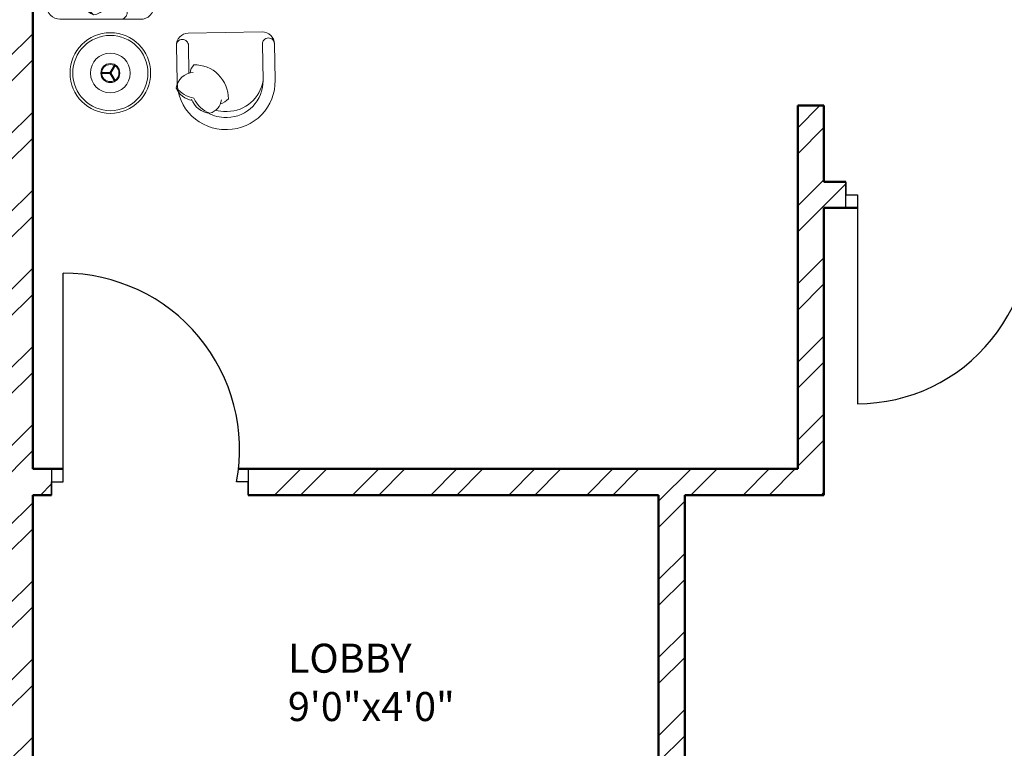
# Model space of a CAD drawing. Units: inches. Extents: x 963 to 2075, y 289 to 2657.
# Tile 82 of 98: x 1511 to 1681, y 2117 to 2243. Entities that reach past the tile are written whole.
import ezdxf

# ---------------------------------------------------------------- set-up
doc = ezdxf.new("R2010")
doc.units = ezdxf.units.IN
for name, color, linetype, lineweight in [('A-AREA-IDEN', 7, 'Continuous', 18), ('A-DOOR', 4, 'Continuous', 25), ('A-FURN', 8, 'Continuous', 18), ('A-WALL', 7, 'Continuous', 50), ('A-WALL-PATT', 8, 'Continuous', 13)]:
    doc.layers.add(name, color=color, linetype=linetype, lineweight=lineweight)
doc.styles.get("Standard").update_dxf_attribs({"font": 'arial.ttf'})

# ---------------------------------------------------------------- blocks, each defined once
blk = doc.blocks.new('ARMCHAIR-A')
at = {"ltscale": 0.03}
blk.add_lwpolyline([(8.89, 17.18), (2.51, 17.18, 0.414214), (0.42, 15.09), (0.42, 8.82, 0.414214), (8.78, 0.46), (8.89, 0.46), (8.99, 0.46, 0.414214), (17.35, 8.82), (17.35, 15.09, 0.414214), (15.26, 17.18), (8.89, 17.18)], format="xyb", dxfattribs=at)
for points in [[(2.51, 8.82), (2.51, 15.09, 0.414214), (1.47, 16.13), (1.47, 16.13, 0.414214), (0.42, 15.09)], [(15.26, 10.28), (15.26, 15.09, -0.414214), (16.31, 16.13), (16.31, 16.13, -0.414214), (17.35, 15.09)], [(15.05, 10.33, 0.165541), (14.41, 11.71, 0.425989), (8.54, 5.73, 0.121523), (9.93, 4.9, -7.115464)], [(14.53, 10.4, -0.356772), (17.52, 7.76, -0.249542), (14.81, 5.59, 9.61688)], [(2.51, 8.82, 0.372719), (8.78, 3.6), (8.89, 3.6)], [(2.51, 8.82, 0.414214), (8.78, 2.55), (8.89, 2.55)], [(17.52, 7.76, -0.14773), (14.47, 5.97, -0.213343), (11.77, 3.34, -0.178662)], [(14.89, 5.83, -0.306663), (11.77, 3.34, -0.30633), (9.74, 5.61, 0.872847)], [(10.77, 3.82, -0.072384), (8.99, 3.6), (8.89, 3.6)], [(12.1, 3.38, -0.130591), (8.99, 2.55), (8.89, 2.55)]]:
    blk.add_lwpolyline(points, format="xyb")
blk = doc.blocks.new('SOFA-3SEAT')
at = {"ltscale": 0.03}
for p, q in [((7.59, 74.33), (6.78, 75.74)), ((7.72, 74.4), (6.9, 75.82)), ((7.59, 74.4), (6.78, 72.99)), ((7.72, 74.33), (6.9, 72.91)), ((7.66, 74.44), (9.29, 74.44)), ((7.66, 74.29), (9.29, 74.29)), ((7.59, 7.12), (6.78, 8.53)), ((7.72, 7.19), (6.9, 8.61)), ((7.59, 7.19), (6.78, 5.78)), ((7.72, 7.12), (6.9, 5.7)), ((7.66, 7.23), (9.29, 7.23)), ((7.66, 7.08), (9.29, 7.08))]:
    blk.add_line(p, q, dxfattribs=at)
blk.add_lwpolyline([(2.44, 16.43, -0.414214), (0.12, 18.74), (0.12, 32.65, -0.414214), (1.28, 33.81, -0.414214), (0.12, 34.97), (0.12, 46.55, -0.414214), (1.28, 47.71, -0.414214), (0.12, 48.87), (0.12, 62.78, -0.414214), (2.44, 65.1), (16.35, 65.1, -0.414214), (18.66, 62.78), (18.66, 18.74, -0.414214), (16.35, 16.43)], format="xyb", close=True, dxfattribs=at)
for points in [[(7.71, 61.62), (5.92, 61.62, -0.414214), (4.76, 62.78), (4.76, 63.94, -0.414214), (5.92, 65.1)], [(7.64, 61.04, -0.356772), (10.56, 64.36, -0.249542), (12.97, 61.35, 9.61688)], [(10.56, 64.36, -0.14773), (12.56, 60.97, -0.213343), (15.48, 57.98, -0.178662)], [(7.71, 61.62, 0.165541), (6.18, 60.9, 0.200231), (8.05, 56.3, 0.121523)], [(12.71, 61.44, -0.306663), (15.48, 57.98, -0.30633), (12.95, 55.72, 0.872847)], [(15.19, 59.18), (15.19, 61.62), (12.91, 61.62, -0.414214)], [(14.03, 60.73), (14.03, 61.16, -0.414214), (14.49, 61.62), (14.72, 61.62, -0.414214), (15.19, 61.16)], [(15.19, 61.16), (15.19, 59.18, -0.414214)], [(7.64, 54.8, -0.356772), (10.56, 58.12, -0.249542), (12.97, 55.11, 9.61688)], [(10.56, 58.12, -0.14773), (12.56, 54.73, -0.213343), (15.48, 51.74, -0.178662)], [(14.03, 54.49), (14.03, 56.09, -0.414214)], [(15.19, 57.25), (15.19, 52.94, -0.414214)], [(7.71, 55.38, 0.165541), (6.18, 54.66, 0.425989), (12.82, 48.15, 0.121523), (13.74, 49.7, -7.115464)], [(12.71, 55.2, -0.306663), (15.48, 51.74, -0.30633), (12.95, 49.48, 0.872847)], [(13.28, 54.97, 0.071865), (13.74, 55.94, -7.115464)], [(15.19, 51.01), (15.19, 48.18, -0.414214), (14.72, 47.71), (14.49, 47.71, -0.414214), (14.03, 48.18), (14.03, 49.84, -0.414214)], [(14.03, 48.87, -0.414214), (12.87, 47.71), (1.28, 47.71, -0.414214)], [(14.03, 46.55, 0.414214), (12.87, 47.71)], [(14.03, 34.97, -0.414214), (12.87, 33.81)], [(14.03, 32.65, 0.414214), (12.87, 33.81), (1.28, 33.81, 0.414214)], [(15.19, 24.27), (15.19, 33.34, 0.414214), (14.72, 33.81), (14.49, 33.81, 0.414214), (14.03, 33.34), (14.03, 25.43, 0.414214)], [(7.71, 19.9, -0.165541), (6.18, 20.62, -0.425989), (12.82, 27.12, -0.121523), (13.74, 25.58, 7.115464)], [(12.71, 20.08, 0.306663), (15.48, 23.54, 0.30633), (12.95, 25.8, -0.872847)], [(10.56, 17.16, 0.14773), (12.56, 20.55, 0.213343), (15.48, 23.54, 0.178662)], [(15.19, 20.37), (15.19, 22.34, 0.414214)], [(7.64, 20.48, 0.356772), (10.56, 17.16, 0.249542), (12.97, 20.17, -9.61688)], [(14.03, 20.79), (14.03, 20.37, 0.414214), (14.49, 19.9), (14.72, 19.9, 0.414214), (15.19, 20.37)], [(5.92, 16.43, -0.414214), (4.76, 17.58), (4.76, 18.74, -0.414214), (5.92, 19.9), (7.71, 19.9)]]:
    blk.add_lwpolyline(points, format="xyb")
for points in [[(15.19, 52.94), (15.19, 57.25)], [(15.19, 24.27), (15.19, 51.01)], [(12.91, 19.9), (15.19, 19.9), (15.19, 22.34)]]:
    blk.add_lwpolyline(points)
blk.add_lwpolyline([(15.19, 47.25), (15.19, 34.27, -0.414214), (14.72, 33.81), (14.49, 33.81, -0.414214), (14.03, 34.27), (14.03, 47.25, -0.414214), (14.49, 47.71), (14.72, 47.71, -0.414214)], format="xyb", close=True)
for centre, radius in [((7.66, 74.37), 6.95), ((7.66, 74.37), 3.42), ((7.66, 74.37), 1.64), ((7.66, 74.37), 1.47), ((7.66, 7.16), 6.95), ((7.66, 7.16), 3.42), ((7.66, 7.16), 1.64), ((7.66, 7.16), 1.47)]:
    blk.add_circle(centre, radius, dxfattribs=at)
for centre in [(7.66, 74.37), (7.66, 7.16)]:
    blk.add_circle(centre, 6.49)

msp = doc.modelspace()

# ---------------------------------------------------------------- hatches: boundary and pattern name
at = {"layer": 'A-WALL-PATT'}
h = msp.add_hatch(dxfattribs=at)
h.set_pattern_fill('ANSI32', color=256)
h.paths.add_polyline_path([(1296.92, 2558.32), (1203.92, 2558.32), (1203.92, 2493.82), (1191.53, 2493.82), (1191.53, 2489.32), (1211.06, 2489.32), (1211.06, 2492.02), (1211.06, 2493.82), (1208.42, 2493.82), (1208.42, 2553.82), (1292.42, 2553.82), (1292.42, 2538.86), (1296.92, 2538.86)])
h.paths.add_polyline_path([(1442.42, 2558.32), (1349.42, 2558.32), (1349.42, 2538.94), (1353.92, 2538.94), (1353.92, 2553.82), (1437.92, 2553.82), (1437.92, 2493.82), (1434.54, 2493.82), (1434.54, 2489.32), (1448.31, 2489.32), (1448.31, 2491.57), (1448.31, 2493.82), (1442.42, 2493.82)])
h.paths.add_polyline_path([(1415.55, 2491.57), (1415.55, 2493.82), (1340.94, 2493.82), (1340.94, 2489.32), (1371.92, 2489.32), (1371.92, 2378.32), (1367.6, 2378.32), (1367.6, 2373.82), (1371.92, 2373.82), (1371.92, 2355.19), (1376.42, 2355.19), (1376.42, 2489.32), (1415.55, 2489.32)])
h.paths.add_polyline_path([(1304.94, 2491.57), (1304.94, 2493.82), (1296.92, 2493.82), (1296.92, 2514.86), (1292.42, 2514.86), (1292.42, 2493.82), (1232.81, 2493.82), (1232.81, 2489.32), (1256.42, 2489.32), (1256.42, 2327.32), (1253.71, 2327.32), (1253.71, 2322.82), (1328.42, 2322.82), (1328.42, 2331.15), (1323.92, 2331.15), (1323.92, 2327.32), (1260.92, 2327.32), (1260.92, 2373.82), (1323.92, 2373.82), (1323.92, 2357.81), (1328.42, 2357.81), (1328.42, 2373.82), (1346.01, 2373.82), (1346.01, 2376.07), (1346.01, 2378.32), (1260.92, 2378.32), (1260.92, 2489.32), (1304.94, 2489.32)])
h.paths.add_polyline_path([(1226.65, 2327.32), (1124.42, 2327.32), (1124.42, 2347.45), (1119.92, 2347.45), (1119.92, 2322.82), (1163.42, 2322.82), (1163.42, 2305.43), (1165.67, 2305.43), (1167.92, 2305.43), (1167.92, 2322.82), (1226.65, 2322.82), (1226.65, 2325.07)])
h.paths.add_polyline_path([(1095.92, 2489.32), (1124.42, 2489.32), (1131.53, 2489.32), (1131.53, 2491.57), (1131.53, 2493.82), (1119.92, 2493.82), (1091.42, 2493.82), (1091.42, 2417.32), (1095.92, 2417.32), (1119.92, 2417.32), (1119.92, 2407.45), (1124.42, 2407.45), (1124.42, 2421.82), (1095.92, 2421.82)])
h.paths.add_polyline_path([(1512.92, 2558.32), (1508.42, 2558.32), (1508.42, 2493.82), (1503.4, 2493.82), (1503.4, 2489.32), (1508.42, 2489.32), (1508.42, 2327.32), (1376.42, 2327.32), (1376.42, 2330.27), (1371.92, 2330.27), (1371.92, 2298.74), (1376.42, 2298.74), (1376.42, 2322.82), (1508.42, 2322.82), (1508.42, 2165.32), (1504.26, 2165.32), (1504.26, 2160.82), (1508.42, 2160.82), (1508.42, 2108.32), (1512.92, 2108.32), (1512.92, 2160.82), (1516.18, 2160.82), (1516.18, 2163.07), (1516.18, 2165.32), (1512.92, 2165.32), (1512.92, 2322.82), (1644.92, 2322.82), (1644.92, 2298.74), (1649.42, 2298.74), (1649.42, 2322.82), (1649.42, 2330.94), (1647.17, 2330.94), (1644.92, 2330.94), (1644.92, 2327.32), (1512.92, 2327.32), (1512.92, 2489.32), (1516.76, 2489.32), (1516.76, 2491.57), (1516.76, 2493.82), (1512.92, 2493.82)])
h.paths.add_polyline_path([(1671.92, 2558.32), (1578.92, 2558.32), (1578.92, 2493.82), (1573.53, 2493.82), (1573.53, 2489.32), (1586.54, 2489.32), (1586.54, 2491.57), (1586.54, 2493.82), (1583.42, 2493.82), (1583.42, 2553.82), (1667.42, 2553.82), (1667.42, 2541.11), (1671.92, 2541.11)])
h.paths.add_polyline_path([(1681.26, 2493.82), (1671.92, 2493.82), (1671.92, 2517.11), (1667.42, 2517.11), (1667.42, 2493.82), (1610.22, 2493.82), (1610.22, 2489.32), (1644.92, 2489.32), (1644.92, 2357.87), (1649.42, 2357.87), (1649.42, 2373.82), (1652.2, 2373.82), (1652.2, 2375.83), (1652.2, 2378.32), (1649.42, 2378.32), (1649.42, 2489.32), (1681.26, 2489.32), (1681.26, 2491.57)])
h.paths.add_polyline_path([(1821.92, 2558.32), (1728.92, 2558.32), (1728.92, 2541), (1733.42, 2541), (1733.42, 2553.82), (1817.42, 2553.82), (1817.42, 2493.82), (1813.51, 2493.82), (1813.51, 2489.32), (1830.08, 2489.32), (1830.08, 2491.57), (1830.08, 2493.82), (1821.92, 2493.82)])
h.paths.add_polyline_path([(1794.24, 2493.82), (1717.26, 2493.82), (1717.26, 2489.32), (1760.42, 2489.32), (1760.42, 2378.32), (1674.4, 2378.32), (1674.4, 2373.82), (1692.92, 2373.82), (1692.92, 2356.95), (1697.42, 2356.95), (1697.42, 2373.82), (1760.42, 2373.82), (1760.42, 2327.32), (1697.42, 2327.32), (1697.42, 2333.34), (1692.92, 2333.34), (1692.92, 2322.82), (1768.04, 2322.82), (1768.04, 2325.07), (1768.04, 2327.32), (1764.92, 2327.32), (1764.92, 2489.32), (1794.24, 2489.32)])
h.paths.add_polyline_path([(1733.42, 2517), (1728.92, 2517), (1728.92, 2493.82), (1733.42, 2493.82)], flags=17)
h.paths.add_polyline_path([(1929.92, 2493.82), (1890.08, 2493.82), (1890.08, 2489.32), (1896.92, 2489.32), (1925.42, 2489.32), (1925.42, 2421.82), (1896.92, 2421.82), (1896.92, 2408.32), (1901.42, 2408.32), (1901.42, 2417.32), (1925.42, 2417.32), (1929.92, 2417.32)])
h.paths.add_polyline_path([(1901.42, 2348.32), (1896.92, 2348.32), (1896.92, 2327.32), (1800.42, 2327.32), (1800.42, 2322.82), (1853.42, 2322.82), (1853.42, 2309.45), (1857.92, 2309.45), (1857.92, 2322.82), (1901.42, 2322.82)])
h.paths.add_polyline_path([(1857.92, 2249.45), (1853.42, 2249.45), (1853.42, 2214.82), (1686.31, 2214.82), (1686.31, 2210.32), (1853.42, 2210.32), (1853.42, 2202.13), (1857.92, 2202.13), (1857.92, 2210.32)])
h.paths.add_polyline_path([(1857.92, 2142.13), (1853.42, 2142.13), (1853.42, 2115.42), (1841.42, 2115.42), (1841.42, 2088.53), (1841.42, 2046.95), (1845.92, 2046.95), (1845.92, 2110.92), (1905.92, 2110.92), (1905.92, 2092.52), (1910.42, 2092.52), (1910.42, 2115.42), (1857.92, 2115.42)])
h.paths.add_polyline_path([(1532.44, 1482.34), (1573.46, 1482.34), (1573.46, 1501), (1532.44, 1501)], flags=9)
h.paths.add_polyline_path([(1438.66, 1486.3), (1479.68, 1486.3), (1479.68, 1504.96), (1438.66, 1504.96)], flags=9)
h.paths.add_polyline_path([(1411.22, 1365.31), (1659.14, 1365.31), (1659.14, 1402.4), (1411.22, 1402.4)], flags=9)
h.paths.add_polyline_path([(1185.67, 2296.3), (1248.16, 2296.3), (1248.16, 2314.95), (1185.67, 2314.95)], flags=9)
h.paths.add_polyline_path([(1177.31, 2187.35), (1216.15, 2187.35), (1216.15, 2206.01), (1177.31, 2206.01)], flags=9)
h.paths.add_polyline_path([(1295.1, 1602.08), (1328.26, 1602.08), (1328.26, 1620.74), (1295.1, 1620.74)], flags=9)
h.paths.add_polyline_path([(1525.13, 2005.99), (1558.39, 2005.99), (1558.39, 2024.65), (1525.13, 2024.65)], flags=9)
h.paths.add_polyline_path([(1459.61, 1977.13), (1472.19, 1977.13), (1472.19, 1987.43), (1459.61, 1987.43)], flags=9)
h.paths.add_polyline_path([(1467.81, 2053.68), (1480.02, 2053.68), (1480.02, 2063.98), (1467.81, 2063.98)], flags=9)
h.paths.add_polyline_path([(1555.18, 2119.02), (1584.56, 2119.02), (1584.56, 2137.68), (1555.18, 2137.68)], flags=25)
h.paths.add_polyline_path([(1405.39, 2115.29), (1444.48, 2115.29), (1444.48, 2133.95), (1405.39, 2133.95)], flags=25)
h.paths.add_polyline_path([(1698.48, 2004.26), (1727.69, 2004.26), (1727.69, 2022.92), (1698.48, 2022.92)], flags=9)
h.paths.add_polyline_path([(1612.16, 1972.86), (1629.02, 1972.86), (1629.02, 1983.16), (1612.16, 1983.16)], flags=9)
h.paths.add_polyline_path([(1608.29, 2060.04), (1625.15, 2060.04), (1625.15, 2070.34), (1608.29, 2070.34)], flags=9)
h.paths.add_polyline_path([(1527.95, 1684.4), (1566.79, 1684.4), (1566.79, 1703.06), (1527.95, 1703.06)], flags=9)
h.paths.add_polyline_path([(1422.79, 1683.59), (1461.63, 1683.59), (1461.63, 1702.25), (1422.79, 1702.25)], flags=9)
h.paths.add_polyline_path([(1531.26, 1732.46), (1574.01, 1732.46), (1574.01, 1751.12), (1531.26, 1751.12)], flags=9)
h.paths.add_polyline_path([(1402.87, 1732.85), (1439.8, 1732.85), (1439.8, 1751.5), (1402.87, 1751.5)], flags=9)
h.paths.add_polyline_path([(1243.12, 1923.13), (1281.96, 1923.13), (1281.96, 1941.79), (1243.12, 1941.79)], flags=9)
h.paths.add_polyline_path([(1181.75, 1792.27), (1244.24, 1792.27), (1244.24, 1810.93), (1181.75, 1810.93)], flags=9)
h.paths.add_polyline_path([(1265.82, 1670.3), (1316.07, 1670.3), (1316.07, 1688.96), (1265.82, 1688.96)], flags=9)
h.paths.add_polyline_path([(1140.26, 1676.05), (1179.1, 1676.05), (1179.1, 1694.71), (1140.26, 1694.71)], flags=9)
h.paths.add_polyline_path([(1107.49, 1490.89), (1143.37, 1490.89), (1143.37, 1509.55), (1107.49, 1509.55)], flags=9)
h.paths.add_polyline_path([(1217.58, 1483.9), (1246.74, 1483.9), (1246.74, 1502.56), (1217.58, 1502.56)], flags=9)
h.paths.add_polyline_path([(1389.21, 1486.92), (1418.37, 1486.92), (1418.37, 1505.58), (1389.21, 1505.58)], flags=9)
h.paths.add_polyline_path([(1672.21, 1602.08), (1705.37, 1602.08), (1705.37, 1620.74), (1672.21, 1620.74)], flags=9)
h.paths.add_polyline_path([(1752.08, 1522.64), (1781.24, 1522.64), (1781.24, 1541.3), (1752.08, 1541.3)], flags=9)
h.paths.add_polyline_path([(1848.27, 1491.26), (1884.16, 1491.26), (1884.16, 1509.92), (1848.27, 1509.92)], flags=9)
h.paths.add_polyline_path([(1822.47, 1685.62), (1861.31, 1685.62), (1861.31, 1704.28), (1822.47, 1704.28)], flags=9)
h.paths.add_polyline_path([(1713.19, 1672.23), (1763.44, 1672.23), (1763.44, 1690.89), (1713.19, 1690.89)], flags=9)
h.paths.add_polyline_path([(1736.62, 1790.58), (1799.11, 1790.58), (1799.11, 1809.24), (1736.62, 1809.24)], flags=9)
h.paths.add_polyline_path([(1691.49, 1916.36), (1730.33, 1916.36), (1730.33, 1935.01), (1691.49, 1935.01)], flags=9)
h.paths.add_polyline_path([(1764.87, 1973.92), (1794.31, 1973.92), (1794.31, 1992.58), (1764.87, 1992.58)], flags=9)
h.paths.add_polyline_path([(1767.85, 2034.02), (1797.29, 2034.02), (1797.29, 2052.67), (1767.85, 2052.67)], flags=9)
h.paths.add_polyline_path([(1851.59, 2060.33), (1880.75, 2060.33), (1880.75, 2078.99), (1851.59, 2078.99)], flags=25)
h.paths.add_polyline_path([(1688.49, 2086.87), (1727.33, 2086.87), (1727.33, 2105.53), (1688.49, 2105.53)], flags=9)
h.paths.add_polyline_path([(1537.74, 2293.58), (1580.49, 2293.58), (1580.49, 2312.24), (1537.74, 2312.24)], flags=25)
h.paths.add_polyline_path([(1425.59, 2296.11), (1468.34, 2296.11), (1468.34, 2314.77), (1425.59, 2314.77)], flags=25)
h.paths.add_polyline_path([(1278.52, 2004.18), (1307.72, 2004.18), (1307.72, 2022.84), (1278.52, 2022.84)], flags=9)
h.paths.add_polyline_path([(1193.28, 1973.63), (1222.72, 1973.63), (1222.72, 1992.29), (1193.28, 1992.29)], flags=9)
h.paths.add_polyline_path([(1192.41, 2040.58), (1221.84, 2040.58), (1221.84, 2059.23), (1192.41, 2059.23)], flags=9)
h.paths.add_polyline_path([(1130.6, 1951.39), (1159.76, 1951.39), (1159.76, 1970.05), (1130.6, 1970.05)], flags=9)
h.paths.add_polyline_path([(1132.83, 2052.49), (1161.98, 2052.49), (1161.98, 2071.15), (1132.83, 2071.15)], flags=9)
h.paths.add_polyline_path([(1265.13, 2334.62), (1315.38, 2334.62), (1315.38, 2353.28), (1265.13, 2353.28)], flags=25)
h.paths.add_polyline_path([(1136.74, 2330.79), (1175.58, 2330.79), (1175.58, 2349.44), (1136.74, 2349.44)], flags=9)
h.paths.add_polyline_path([(1287.42, 2417.2), (1320.58, 2417.2), (1320.58, 2435.86), (1287.42, 2435.86)], flags=25)
h.paths.add_polyline_path([(1430.99, 2329.16), (1469.83, 2329.16), (1469.83, 2347.82), (1430.99, 2347.82)], flags=25)
h.paths.add_polyline_path([(1525.42, 2329.21), (1564.26, 2329.21), (1564.26, 2347.87), (1525.42, 2347.87)], flags=25)
h.paths.add_polyline_path([(1684.52, 2382.8), (1717.68, 2382.8), (1717.68, 2401.46), (1684.52, 2401.46)], flags=25)
h.paths.add_polyline_path([(1704.81, 2340.29), (1755.05, 2340.29), (1755.05, 2358.95), (1704.81, 2358.95)], flags=25)
h.paths.add_polyline_path([(1694.11, 2287.76), (1756.6, 2287.76), (1756.6, 2306.41), (1694.11, 2306.41)], flags=9)
h.paths.add_polyline_path([(1815.78, 2329.86), (1854.62, 2329.86), (1854.62, 2348.52), (1815.78, 2348.52)], flags=9)
h.paths.add_polyline_path([(1842.87, 2514.26), (1878.76, 2514.26), (1878.76, 2532.91), (1842.87, 2532.91)], flags=9)
h.paths.add_polyline_path([(1769.51, 2531.45), (1798.67, 2531.45), (1798.67, 2550.1), (1769.51, 2550.1)], flags=25)
h.paths.add_polyline_path([(1594.77, 2518.47), (1623.93, 2518.47), (1623.93, 2537.13), (1594.77, 2537.13)], flags=25)
h.paths.add_polyline_path([(1520.72, 2516.18), (1556.61, 2516.18), (1556.61, 2534.84), (1520.72, 2534.84)], flags=25)
h.paths.add_polyline_path([(1464.46, 2516.69), (1500.34, 2516.69), (1500.34, 2535.35), (1464.46, 2535.35)], flags=25)
h.paths.add_polyline_path([(1365.7, 2528.97), (1394.85, 2528.97), (1394.85, 2547.63), (1365.7, 2547.63)], flags=25)
h.paths.add_polyline_path([(1222.84, 2516.23), (1252, 2516.23), (1252, 2534.89), (1222.84, 2534.89)], flags=25)
h.paths.add_polyline_path([(1104.55, 2509.6), (1140.43, 2509.6), (1140.43, 2528.26), (1104.55, 2528.26)], flags=9)
h = msp.add_hatch(dxfattribs=at)
h.set_pattern_fill('ANSI32', color=256)
h.paths.add_polyline_path([(1335.97, 2212.57), (1335.97, 2214.82), (1167.92, 2214.82), (1167.92, 2245.43), (1163.42, 2245.43), (1163.42, 2210.32), (1163.42, 2194.81), (1167.92, 2194.81), (1167.92, 2210.32), (1335.97, 2210.32)])
h.paths.add_polyline_path([(1532.44, 1482.34), (1573.46, 1482.34), (1573.46, 1501), (1532.44, 1501)], flags=9)
h.paths.add_polyline_path([(1438.66, 1486.3), (1479.68, 1486.3), (1479.68, 1504.96), (1438.66, 1504.96)], flags=9)
h.paths.add_polyline_path([(1411.22, 1365.31), (1659.14, 1365.31), (1659.14, 1402.4), (1411.22, 1402.4)], flags=9)
h.paths.add_polyline_path([(1185.67, 2296.3), (1248.16, 2296.3), (1248.16, 2314.95), (1185.67, 2314.95)], flags=9)
h.paths.add_polyline_path([(1177.31, 2187.35), (1216.15, 2187.35), (1216.15, 2206.01), (1177.31, 2206.01)], flags=9)
h.paths.add_polyline_path([(1295.1, 1602.08), (1328.26, 1602.08), (1328.26, 1620.74), (1295.1, 1620.74)], flags=9)
h.paths.add_polyline_path([(1525.13, 2005.99), (1558.39, 2005.99), (1558.39, 2024.65), (1525.13, 2024.65)], flags=9)
h.paths.add_polyline_path([(1459.61, 1977.13), (1472.19, 1977.13), (1472.19, 1987.43), (1459.61, 1987.43)], flags=9)
h.paths.add_polyline_path([(1467.81, 2053.68), (1480.02, 2053.68), (1480.02, 2063.98), (1467.81, 2063.98)], flags=9)
h.paths.add_polyline_path([(1555.18, 2119.02), (1584.56, 2119.02), (1584.56, 2137.68), (1555.18, 2137.68)], flags=9)
h.paths.add_polyline_path([(1405.39, 2115.29), (1444.48, 2115.29), (1444.48, 2133.95), (1405.39, 2133.95)], flags=9)
h.paths.add_polyline_path([(1698.48, 2004.26), (1727.69, 2004.26), (1727.69, 2022.92), (1698.48, 2022.92)], flags=9)
h.paths.add_polyline_path([(1612.16, 1972.86), (1629.02, 1972.86), (1629.02, 1983.16), (1612.16, 1983.16)], flags=9)
h.paths.add_polyline_path([(1608.29, 2060.04), (1625.15, 2060.04), (1625.15, 2070.34), (1608.29, 2070.34)], flags=9)
h.paths.add_polyline_path([(1527.95, 1684.4), (1566.79, 1684.4), (1566.79, 1703.06), (1527.95, 1703.06)], flags=9)
h.paths.add_polyline_path([(1422.79, 1683.59), (1461.63, 1683.59), (1461.63, 1702.25), (1422.79, 1702.25)], flags=9)
h.paths.add_polyline_path([(1531.26, 1732.46), (1574.01, 1732.46), (1574.01, 1751.12), (1531.26, 1751.12)], flags=9)
h.paths.add_polyline_path([(1402.87, 1732.85), (1439.8, 1732.85), (1439.8, 1751.5), (1402.87, 1751.5)], flags=9)
h.paths.add_polyline_path([(1243.12, 1923.13), (1281.96, 1923.13), (1281.96, 1941.79), (1243.12, 1941.79)], flags=9)
h.paths.add_polyline_path([(1181.75, 1792.27), (1244.24, 1792.27), (1244.24, 1810.93), (1181.75, 1810.93)], flags=9)
h.paths.add_polyline_path([(1265.82, 1670.3), (1316.07, 1670.3), (1316.07, 1688.96), (1265.82, 1688.96)], flags=9)
h.paths.add_polyline_path([(1140.26, 1676.05), (1179.1, 1676.05), (1179.1, 1694.71), (1140.26, 1694.71)], flags=9)
h.paths.add_polyline_path([(1107.49, 1490.89), (1143.37, 1490.89), (1143.37, 1509.55), (1107.49, 1509.55)], flags=9)
h.paths.add_polyline_path([(1217.58, 1483.9), (1246.74, 1483.9), (1246.74, 1502.56), (1217.58, 1502.56)], flags=9)
h.paths.add_polyline_path([(1389.21, 1486.92), (1418.37, 1486.92), (1418.37, 1505.58), (1389.21, 1505.58)], flags=9)
h.paths.add_polyline_path([(1672.21, 1602.08), (1705.37, 1602.08), (1705.37, 1620.74), (1672.21, 1620.74)], flags=9)
h.paths.add_polyline_path([(1752.08, 1522.64), (1781.24, 1522.64), (1781.24, 1541.3), (1752.08, 1541.3)], flags=9)
h.paths.add_polyline_path([(1848.27, 1491.26), (1884.16, 1491.26), (1884.16, 1509.92), (1848.27, 1509.92)], flags=9)
h.paths.add_polyline_path([(1822.47, 1685.62), (1861.31, 1685.62), (1861.31, 1704.28), (1822.47, 1704.28)], flags=9)
h.paths.add_polyline_path([(1713.19, 1672.23), (1763.44, 1672.23), (1763.44, 1690.89), (1713.19, 1690.89)], flags=9)
h.paths.add_polyline_path([(1736.62, 1790.58), (1799.11, 1790.58), (1799.11, 1809.24), (1736.62, 1809.24)], flags=9)
h.paths.add_polyline_path([(1691.49, 1916.36), (1730.33, 1916.36), (1730.33, 1935.01), (1691.49, 1935.01)], flags=9)
h.paths.add_polyline_path([(1764.87, 1973.92), (1794.31, 1973.92), (1794.31, 1992.58), (1764.87, 1992.58)], flags=9)
h.paths.add_polyline_path([(1767.85, 2034.02), (1797.29, 2034.02), (1797.29, 2052.67), (1767.85, 2052.67)], flags=9)
h.paths.add_polyline_path([(1851.59, 2060.33), (1880.75, 2060.33), (1880.75, 2078.99), (1851.59, 2078.99)], flags=9)
h.paths.add_polyline_path([(1688.49, 2086.87), (1727.33, 2086.87), (1727.33, 2105.53), (1688.49, 2105.53)], flags=9)
h.paths.add_polyline_path([(1537.74, 2293.58), (1580.49, 2293.58), (1580.49, 2312.24), (1537.74, 2312.24)], flags=9)
h.paths.add_polyline_path([(1425.59, 2296.11), (1468.34, 2296.11), (1468.34, 2314.77), (1425.59, 2314.77)], flags=9)
h.paths.add_polyline_path([(1278.52, 2004.18), (1307.72, 2004.18), (1307.72, 2022.84), (1278.52, 2022.84)], flags=9)
h.paths.add_polyline_path([(1193.28, 1973.63), (1222.72, 1973.63), (1222.72, 1992.29), (1193.28, 1992.29)], flags=9)
h.paths.add_polyline_path([(1192.41, 2040.58), (1221.84, 2040.58), (1221.84, 2059.23), (1192.41, 2059.23)], flags=9)
h.paths.add_polyline_path([(1130.6, 1951.39), (1159.76, 1951.39), (1159.76, 1970.05), (1130.6, 1970.05)], flags=9)
h.paths.add_polyline_path([(1132.83, 2052.49), (1161.98, 2052.49), (1161.98, 2071.15), (1132.83, 2071.15)], flags=9)
h.paths.add_polyline_path([(1265.13, 2334.62), (1315.38, 2334.62), (1315.38, 2353.28), (1265.13, 2353.28)], flags=9)
h.paths.add_polyline_path([(1136.74, 2330.79), (1175.58, 2330.79), (1175.58, 2349.44), (1136.74, 2349.44)], flags=9)
h.paths.add_polyline_path([(1287.42, 2417.2), (1320.58, 2417.2), (1320.58, 2435.86), (1287.42, 2435.86)], flags=9)
h.paths.add_polyline_path([(1430.99, 2329.16), (1469.83, 2329.16), (1469.83, 2347.82), (1430.99, 2347.82)], flags=9)
h.paths.add_polyline_path([(1525.42, 2329.21), (1564.26, 2329.21), (1564.26, 2347.87), (1525.42, 2347.87)], flags=9)
h.paths.add_polyline_path([(1684.52, 2382.8), (1717.68, 2382.8), (1717.68, 2401.46), (1684.52, 2401.46)], flags=9)
h.paths.add_polyline_path([(1704.81, 2340.29), (1755.05, 2340.29), (1755.05, 2358.95), (1704.81, 2358.95)], flags=9)
h.paths.add_polyline_path([(1694.11, 2287.76), (1756.6, 2287.76), (1756.6, 2306.41), (1694.11, 2306.41)], flags=9)
h.paths.add_polyline_path([(1815.78, 2329.86), (1854.62, 2329.86), (1854.62, 2348.52), (1815.78, 2348.52)], flags=9)
h.paths.add_polyline_path([(1842.87, 2514.26), (1878.76, 2514.26), (1878.76, 2532.91), (1842.87, 2532.91)], flags=9)
h.paths.add_polyline_path([(1769.51, 2531.45), (1798.67, 2531.45), (1798.67, 2550.1), (1769.51, 2550.1)], flags=9)
h.paths.add_polyline_path([(1594.77, 2518.47), (1623.93, 2518.47), (1623.93, 2537.13), (1594.77, 2537.13)], flags=9)
h.paths.add_polyline_path([(1520.72, 2516.18), (1556.61, 2516.18), (1556.61, 2534.84), (1520.72, 2534.84)], flags=9)
h.paths.add_polyline_path([(1464.46, 2516.69), (1500.34, 2516.69), (1500.34, 2535.35), (1464.46, 2535.35)], flags=9)
h.paths.add_polyline_path([(1365.7, 2528.97), (1394.85, 2528.97), (1394.85, 2547.63), (1365.7, 2547.63)], flags=9)
h.paths.add_polyline_path([(1222.84, 2516.23), (1252, 2516.23), (1252, 2534.89), (1222.84, 2534.89)], flags=9)
h.paths.add_polyline_path([(1104.55, 2509.6), (1140.43, 2509.6), (1140.43, 2528.26), (1104.55, 2528.26)], flags=9)
h = msp.add_hatch(dxfattribs=at)
h.set_pattern_fill('ANSI32', color=256)
h.paths.add_polyline_path([(1473.61, 2163.07), (1473.61, 2165.32), (1376.42, 2165.32), (1376.42, 2227.98), (1371.92, 2227.98), (1371.92, 2214.82), (1368.41, 2214.82), (1368.41, 2210.32), (1371.92, 2210.32), (1371.92, 2160.82), (1395.92, 2160.82), (1395.92, 2090.32), (1217.34, 2090.32), (1217.34, 2085.82), (1395.92, 2085.82), (1458.92, 2085.82), (1458.92, 2108.32), (1454.42, 2108.32), (1454.42, 2090.32), (1400.42, 2090.32), (1400.42, 2160.82), (1473.61, 2160.82)])
h.paths.add_polyline_path([(1649.42, 2210.32), (1653.23, 2210.32), (1653.23, 2214.82), (1649.42, 2214.82), (1649.42, 2227.98), (1644.92, 2227.98), (1644.92, 2165.32), (1550.1, 2165.32), (1550.1, 2160.82), (1620.92, 2160.82), (1620.92, 2112.82), (1555.45, 2112.82), (1555.45, 2108.32), (1584.33, 2108.32), (1584.33, 2084.92), (1588.83, 2084.92), (1588.83, 2108.32), (1625.42, 2108.32), (1667.95, 2108.32), (1667.95, 2022.67), (1588.83, 2022.67), (1588.83, 2047.41), (1584.33, 2047.41), (1584.33, 1996), (1588.83, 1996), (1588.83, 2018.32), (1667.95, 2018.17), (1667.95, 1928.32), (1625.42, 1928.32), (1625.42, 1923.82), (1672.45, 1923.82), (1672.45, 1928.32), (1672.45, 1946.66), (1785.45, 1946.66), (1785.45, 1951.16), (1743.03, 1951.16), (1743.03, 2017.92), (1841.42, 2017.92), (1841.42, 2014.77), (1845.92, 2014.77), (1845.92, 2017.92), (1905.92, 2017.92), (1905.92, 1987.51), (1910.42, 1987.51), (1910.42, 2022.42), (1910.42, 2068.52), (1905.92, 2068.52), (1905.92, 2022.42), (1845.92, 2022.42), (1845.92, 2025.85), (1843.67, 2025.85), (1841.42, 2025.85), (1841.42, 2022.42), (1743.03, 2022.42), (1743.03, 2084.03), (1768.45, 2084.03), (1785.45, 2084.03), (1785.45, 2088.53), (1672.45, 2088.53), (1672.45, 2112.82), (1667.95, 2112.82), (1625.42, 2112.82), (1625.42, 2160.82), (1649.42, 2160.82)])
h.paths.add_polyline_path([(1672.45, 2084.03), (1738.53, 2084.03), (1738.53, 1951.16), (1672.45, 1951.16)], flags=16)
h.paths.add_polyline_path([(1672.45, 2084.03), (1738.53, 2084.03), (1705.49, 2017.6)], flags=0)
h.paths.add_polyline_path([(1262.77, 2085.82), (1258.27, 2085.82), (1258.27, 2023.28), (1184.42, 2023.28), (1184.42, 2018.78), (1258.27, 2018.78), (1258.27, 1950.82), (1262.77, 1950.82)])
h.paths.add_polyline_path([(1312.27, 2085.82), (1307.77, 2085.82), (1307.77, 1950.82), (1312.27, 1950.82)])
h.paths.add_polyline_path([(1458.92, 1950.82), (1395.92, 1950.82), (1216.57, 1950.82), (1216.57, 1946.32), (1346.42, 1946.32), (1395.92, 1946.32), (1395.92, 1875.82), (1371.92, 1875.82), (1371.92, 1826.32), (1368.93, 1826.32), (1368.93, 1821.82), (1371.92, 1821.82), (1371.92, 1813.62), (1376.42, 1813.62), (1376.42, 1871.32), (1474.5, 1871.32), (1474.5, 1873.57), (1474.5, 1875.82), (1400.42, 1875.82), (1400.42, 1946.32), (1454.42, 1946.32), (1454.42, 1928.32), (1458.92, 1928.32)])
h.paths.add_polyline_path([(1184.42, 2120.78), (1167.92, 2120.78), (1167.92, 2134.81), (1165.67, 2134.81), (1163.42, 2134.81), (1163.42, 2120.78), (1119.92, 2120.78), (1119.92, 2098.1), (1124.42, 2098.1), (1124.42, 2116.28), (1167.92, 2116.28), (1179.92, 2116.28), (1179.92, 2045.92), (1184.42, 2045.92), (1184.42, 2090.32), (1184.42, 2116.28)])
h.paths.add_polyline_path([(1124.42, 2018.78), (1179.92, 2018.78), (1179.92, 2016.29), (1184.42, 2016.29), (1184.42, 2023.28), (1184.42, 2026.59), (1182.17, 2026.59), (1179.92, 2026.59), (1179.92, 2023.28), (1124.42, 2023.28), (1124.42, 2074.1), (1119.92, 2074.1), (1119.92, 2018.78), (1119.92, 1979.63), (1124.42, 1979.63)])
h.paths.add_polyline_path([(1184.42, 1925.78), (1184.42, 1946.32), (1184.42, 1996.07), (1182.17, 1996.07), (1179.92, 1996.07), (1179.92, 1925.78), (1124.42, 1925.78), (1124.42, 1955.63), (1119.92, 1955.5), (1119.92, 1921.28), (1158.92, 1921.28), (1158.92, 1909.98), (1163.42, 1909.98), (1163.42, 1921.28), (1184.42, 1921.28)])
h.paths.add_polyline_path([(1341.45, 1826.32), (1163.42, 1826.32), (1163.42, 1849.98), (1158.92, 1849.98), (1158.92, 1821.82), (1158.92, 1804.03), (1163.42, 1804.03), (1163.42, 1821.82), (1341.45, 1821.82)])
h.paths.add_polyline_path([(1222.98, 1713.82), (1163.42, 1713.82), (1163.42, 1744.03), (1161.17, 1744.03), (1158.92, 1744.03), (1158.92, 1713.82), (1119.92, 1713.82), (1119.92, 1694.65), (1124.42, 1694.65), (1124.42, 1709.32), (1158.92, 1709.32), (1222.98, 1709.32)])
h.paths.add_polyline_path([(1328.42, 1713.82), (1252.04, 1713.82), (1252.04, 1711.57), (1252.04, 1709.32), (1256.42, 1709.32), (1256.42, 1547.32), (1232.94, 1547.32), (1232.94, 1545.07), (1232.94, 1542.82), (1292.42, 1542.82), (1292.42, 1527.63), (1296.92, 1527.63), (1296.92, 1542.82), (1299.46, 1542.82), (1299.46, 1547.32), (1260.92, 1547.32), (1260.92, 1658.32), (1343.66, 1658.32), (1343.66, 1660.57), (1343.66, 1662.82), (1328.42, 1662.82), (1328.42, 1676.59), (1327.4, 1676.59), (1323.92, 1676.59), (1323.92, 1662.82), (1260.92, 1662.82), (1260.92, 1709.32), (1323.92, 1709.32), (1323.92, 1699.85), (1328.42, 1699.85)])
h.paths.add_polyline_path([(1649.42, 1875.82), (1625.42, 1875.82), (1625.42, 1928.32), (1620.92, 1928.32), (1588.83, 1928.32), (1588.83, 1950.59), (1584.33, 1950.59), (1584.33, 1928.32), (1555.45, 1928.32), (1555.45, 1923.82), (1620.92, 1923.82), (1620.92, 1875.82), (1548.95, 1875.82), (1548.95, 1873.57), (1548.95, 1871.32), (1644.92, 1871.32), (1644.92, 1813.62), (1649.42, 1813.62), (1649.42, 1821.82), (1652.04, 1821.82), (1652.04, 1824.07), (1652.04, 1826.32), (1649.42, 1826.32)])
h.paths.add_polyline_path([(1512.92, 1871.32), (1516.48, 1871.32), (1516.48, 1875.82), (1512.92, 1875.82), (1512.92, 1923.82), (1512.92, 1928.32), (1512.92, 1930.83), (1508.42, 1930.83), (1508.42, 1875.82), (1504.41, 1875.82), (1504.41, 1871.32), (1508.42, 1871.32), (1508.42, 1713.82), (1376.42, 1713.82), (1376.42, 1743.32), (1371.92, 1743.32), (1371.92, 1709.32), (1371.92, 1706.01), (1376.42, 1706.01), (1376.42, 1709.32), (1508.42, 1709.32), (1508.42, 1547.32), (1501.87, 1547.32), (1501.87, 1542.82), (1508.42, 1542.82), (1508.42, 1482.82), (1508.42, 1436.32), (1512.92, 1436.32), (1512.92, 1542.82), (1519.32, 1542.82), (1519.32, 1545.07), (1519.32, 1547.32), (1512.92, 1547.32), (1512.92, 1709.32), (1644.92, 1709.32), (1644.92, 1707.55), (1649.42, 1707.55), (1649.42, 1709.32), (1649.42, 1743.32), (1644.92, 1743.32), (1644.92, 1713.82), (1512.92, 1713.82)])
h.paths.add_polyline_path([(1129.88, 1545.07), (1129.88, 1547.32), (1124.42, 1547.32), (1095.92, 1547.32), (1095.92, 1614.82), (1124.42, 1614.82), (1124.42, 1619.32), (1095.92, 1619.32), (1091.42, 1619.32), (1091.42, 1542.82), (1095.92, 1542.82), (1119.92, 1542.82), (1129.88, 1542.82)])
h.paths.add_polyline_path([(1208.42, 1542.82), (1211.74, 1542.82), (1211.74, 1547.32), (1198.85, 1547.32), (1198.85, 1542.82), (1203.92, 1542.82), (1203.92, 1478.32), (1208.42, 1478.32), (1296.92, 1478.32), (1296.92, 1503.63), (1292.42, 1503.63), (1292.42, 1482.82), (1208.42, 1482.82)])
h.paths.add_polyline_path([(1430.42, 1542.82), (1435.7, 1542.82), (1435.7, 1545.07), (1435.7, 1547.32), (1422.66, 1547.32), (1422.66, 1545.07), (1422.66, 1542.82), (1425.92, 1542.82), (1425.92, 1482.86), (1341.92, 1482.86), (1341.92, 1502.73), (1337.42, 1502.73), (1337.42, 1478.36), (1425.92, 1478.36), (1425.92, 1440.82), (1425.92, 1436.32), (1430.42, 1436.32)])
h.paths.add_polyline_path([(1698.48, 2004.26), (1727.69, 2004.26), (1727.69, 2022.92), (1698.48, 2022.92)], flags=8)

# ---------------------------------------------------------------- linework, layer by layer
at = {"layer": 'A-DOOR'}
for p, q in [((1653.23, 2210.32), (1653.23, 2214.82)), ((1653.23, 2214.82), (1653.23, 2212.57)), ((1653.23, 2212.57), (1655.23, 2212.57)), ((1655.23, 2212.57), (1655.23, 2176.57)), ((1518.18, 2163.07), (1518.18, 2199.07)), ((1516.18, 2165.32), (1516.18, 2160.82)), ((1550.1, 2165.32), (1550.1, 2160.82)), ((1516.18, 2160.82), (1516.18, 2163.07)), ((1516.18, 2163.07), (1518.18, 2163.07)), ((1550.1, 2163.07), (1548.1, 2163.07)), ((1550.1, 2160.82), (1550.1, 2163.07))]:
    msp.add_line(p, q, dxfattribs=at)
for centre, radius, start, end in [((1655.23, 2206.32), 29.75, 270, 12.1318), ((1518.18, 2168.64), 30.43, 349.4556, 90)]:
    msp.add_arc(centre, radius, start, end, dxfattribs=at)
at = {"layer": 'A-WALL'}
for p, q in [((1512.92, 2165.32), (1512.92, 2322.82)), ((1644.92, 2227.98), (1649.42, 2227.98)), ((1644.92, 2227.98), (1644.92, 2165.32)), ((1649.42, 2227.98), (1649.42, 2214.82)), ((1649.42, 2214.82), (1653.23, 2214.82)), ((1649.42, 2210.32), (1655.23, 2210.32)), ((1649.42, 2210.32), (1649.42, 2160.82)), ((1512.92, 2165.32), (1518.18, 2165.32)), ((1548.43, 2165.32), (1644.92, 2165.32)), ((1512.92, 2160.82), (1516.18, 2160.82)), ((1512.92, 2108.32), (1512.92, 2160.82)), ((1550.1, 2160.82), (1620.92, 2160.82)), ((1620.92, 2112.82), (1620.92, 2160.82)), ((1625.42, 2112.82), (1625.42, 2160.82)), ((1625.42, 2160.82), (1649.42, 2160.82))]:
    msp.add_line(p, q, dxfattribs=at)

# ---------------------------------------------------------------- block references
at = {"layer": 'A-FURN', "rotation": 179.9690487318625}
msp.add_blockref('SOFA-3SEAT', (1534.01, 2307.94), dxfattribs=at)
at = {"layer": 'A-FURN', "extrusion": (0, 0, -1), "zscale": -1, "rotation": 358.9868193276391}
msp.add_blockref('ARMCHAIR-A', (-1555.32, 2223.52), dxfattribs=at)

# ---------------------------------------------------------------- texts
at = {"layer": 'A-AREA-IDEN', "insert": (1556.95, 2135.19), "char_height": 5, "attachment_point": 1}
msp.add_mtext_dynamic_manual_height_columns('LOBBY\\P9\'0"x4\'0"', width=97.0875, gutter_width=12.5, heights=[0], dxfattribs=at)

doc.saveas('drawing.dxf')
